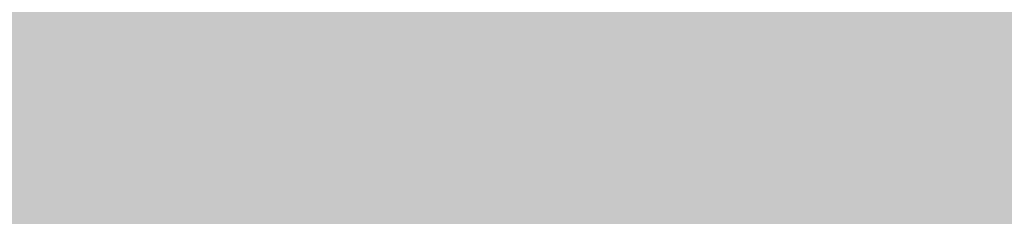
# Model space of a CAD drawing. Units: millimetres. Extents: x -22994 to 29398, y -19990 to 20176.
# Tile 94 of 135: x 229.428 to 230.597, y 84.264 to 84.498. Entities that reach past the tile are written whole.
import ezdxf
from ezdxf import colors
from ezdxf.entities.mleader import LeaderData, LeaderLine
from ezdxf.math import Vec2, Vec3

# ---------------------------------------------------------------- set-up
doc = ezdxf.new("R2010")
doc.units = ezdxf.units.MM
doc.header["$MEASUREMENT"] = 0
for name, color, linetype, lineweight in [('M-ANNO-TEXT', 7, 'Continuous', 25), ('M-DIMS', 2, 'Continuous', 18), ('M-EQPM-PATT', 7, 'Continuous', 18)]:
    doc.layers.add(name, color=color, linetype=linetype, lineweight=lineweight)
doc.styles.get("Standard").update_dxf_attribs({"font": 'arial.ttf'})
doc.dimstyles.get("Standard").update_dxf_attribs({"dimtxt": 0.18, "dimasz": 10000, "dimexe": 0.18, "dimexo": 0.0625, "dimgap": 0.09, "dimtad": 0, "dimtih": 1, "dimtoh": 1, "dimdec": 0, "dimzin": 0, "dimdsep": 46, "dimtxsty": 'Standard', "dimcen": 0.09, "dimadec": 0, "dimazin": 0, "dimtfac": 1, "dimtdec": 0, "dimtofl": 0, "dimtmove": 0, "dimatfit": 3, "dimfxl": 1, "dimtolj": 1, "dimtzin": 0, "dimlwd": 30, "dimarcsym": 0})

# ---------------------------------------------------------------- blocks, each defined once
blk = doc.blocks.new('*D2')
at = {"layer": 'Defpoints', "color": 0, "transparency": 16777216}
for p in [(6.6773, 10.2713), (290.852, 10.2713), (290.852, -5.0787)]:
    blk.add_point(p, dxfattribs=at)
at = {"layer": 'M-DIMS', "color": 0, "lineweight": -2, "transparency": 16777216}
for p, q in [((6.6773, 10.2088), (6.6773, -5.2587)), ((290.852, 10.2088), (290.852, -5.2587))]:
    blk.add_line(p, q, dxfattribs=at)
at = {"layer": 'M-DIMS', "color": 0, "lineweight": 30, "transparency": 16777216}
for p, q in [((-9993.3227, -5.0787), (-19993.3227, -5.0787)), ((10290.852, -5.0787), (20290.852, -5.0787))]:
    blk.add_line(p, q, dxfattribs=at)
at = {"layer": 'M-DIMS', "color": 0, "transparency": 16777216}
for points in [[(-9993.3227, 1661.5879), (-9993.3227, -1671.7454), (6.6773, -5.0787)], [(10290.852, 1661.5879), (10290.852, -1671.7454), (290.852, -5.0787)]]:
    blk.add_solid(points, dxfattribs=at)
at = {"layer": 'M-DIMS', "color": 0, "transparency": 16777216, "insert": (148.7647, -5.0787), "char_height": 0.18, "attachment_point": 5}
blk.add_mtext('\\A1;284.2', dxfattribs=at)
blk = doc.blocks.new('*D3')
at = {"layer": 'Defpoints', "color": 0, "transparency": 16777216}
for p in [(110.2647, 204.1654), (110.2647, 176.3662), (95.8327, 127.967)]:
    blk.add_point(p, dxfattribs=at)
at = {"layer": 'M-DIMS', "color": 0, "lineweight": -2, "transparency": 16777216}
for p, q in [((95.8327, 128.0295), (95.8327, 204.3454)), ((110.2647, 176.4287), (110.2647, 204.3454))]:
    blk.add_line(p, q, dxfattribs=at)
at = {"layer": 'M-DIMS', "color": 0, "lineweight": 30, "transparency": 16777216}
for p, q in [((-9904.1673, 204.1654), (-19904.1673, 204.1654)), ((10110.2647, 204.1654), (20110.2647, 204.1654))]:
    blk.add_line(p, q, dxfattribs=at)
at = {"layer": 'M-DIMS', "color": 0, "transparency": 16777216}
for points in [[(-9904.1673, 1870.8321), (-9904.1673, -1462.5013), (95.8327, 204.1654)], [(10110.2647, 1870.8321), (10110.2647, -1462.5013), (110.2647, 204.1654)]]:
    blk.add_solid(points, dxfattribs=at)
at = {"layer": 'M-DIMS', "color": 0, "transparency": 16777216, "insert": (103.0487, 204.1654), "char_height": 0.18, "attachment_point": 5}
blk.add_mtext('\\A1;14.432', dxfattribs=at)
blk = doc.blocks.new('*D4')
at = {"layer": 'Defpoints', "color": 0, "transparency": 16777216}
for p in [(116.2647, 204.1654), (110.2647, 176.3662), (116.2647, 176.3662)]:
    blk.add_point(p, dxfattribs=at)
at = {"layer": 'M-DIMS', "color": 0, "lineweight": -2, "transparency": 16777216}
for p, q in [((110.2647, 176.4287), (110.2647, 204.3454)), ((116.2647, 176.4287), (116.2647, 204.3454))]:
    blk.add_line(p, q, dxfattribs=at)
at = {"layer": 'M-DIMS', "color": 0, "lineweight": 30, "transparency": 16777216}
for p, q in [((-9889.7353, 204.1654), (-19889.7353, 204.1654)), ((10116.2647, 204.1654), (20116.2647, 204.1654))]:
    blk.add_line(p, q, dxfattribs=at)
at = {"layer": 'M-DIMS', "color": 0, "transparency": 16777216}
for points in [[(-9889.7353, 1870.8321), (-9889.7353, -1462.5013), (110.2647, 204.1654)], [(10116.2647, 1870.8321), (10116.2647, -1462.5013), (116.2647, 204.1654)]]:
    blk.add_solid(points, dxfattribs=at)
at = {"layer": 'M-DIMS', "color": 0, "transparency": 16777216, "insert": (113.2647, 204.1654), "char_height": 0.18, "attachment_point": 5}
blk.add_mtext('\\A1;6', dxfattribs=at)
blk = doc.blocks.new('*D5')
at = {"layer": 'Defpoints', "color": 0, "transparency": 16777216}
for p in [(181.2647, 204.1654), (116.2647, 176.3662), (181.2647, 176.3662)]:
    blk.add_point(p, dxfattribs=at)
at = {"layer": 'M-DIMS', "color": 0, "lineweight": -2, "transparency": 16777216}
for p, q in [((116.2647, 176.4287), (116.2647, 204.3454)), ((181.2647, 176.4287), (181.2647, 204.3454))]:
    blk.add_line(p, q, dxfattribs=at)
at = {"layer": 'M-DIMS', "color": 0, "lineweight": 30, "transparency": 16777216}
for p, q in [((-9883.7353, 204.1654), (-19883.7353, 204.1654)), ((10181.2647, 204.1654), (20181.2647, 204.1654))]:
    blk.add_line(p, q, dxfattribs=at)
at = {"layer": 'M-DIMS', "color": 0, "transparency": 16777216}
for points in [[(-9883.7353, 1870.8321), (-9883.7353, -1462.5013), (116.2647, 204.1654)], [(10181.2647, 1870.8321), (10181.2647, -1462.5013), (181.2647, 204.1654)]]:
    blk.add_solid(points, dxfattribs=at)
at = {"layer": 'M-DIMS', "color": 0, "transparency": 16777216, "insert": (148.7647, 204.1654), "char_height": 0.18, "attachment_point": 5}
blk.add_mtext('\\A1;65', dxfattribs=at)
blk = doc.blocks.new('*D6')
at = {"layer": 'Defpoints', "color": 0, "transparency": 16777216}
for p in [(187.2647, 204.1654), (181.2647, 176.3662), (187.2647, 176.3662)]:
    blk.add_point(p, dxfattribs=at)
at = {"layer": 'M-DIMS', "color": 0, "lineweight": -2, "transparency": 16777216}
for p, q in [((181.2647, 176.4287), (181.2647, 204.3454)), ((187.2647, 176.4287), (187.2647, 204.3454))]:
    blk.add_line(p, q, dxfattribs=at)
at = {"layer": 'M-DIMS', "color": 0, "lineweight": 30, "transparency": 16777216}
for p, q in [((-9818.7353, 204.1654), (-19818.7353, 204.1654)), ((10187.2647, 204.1654), (20187.2647, 204.1654))]:
    blk.add_line(p, q, dxfattribs=at)
at = {"layer": 'M-DIMS', "color": 0, "transparency": 16777216}
for points in [[(-9818.7353, 1870.8321), (-9818.7353, -1462.5013), (181.2647, 204.1654)], [(10187.2647, 1870.8321), (10187.2647, -1462.5013), (187.2647, 204.1654)]]:
    blk.add_solid(points, dxfattribs=at)
at = {"layer": 'M-DIMS', "color": 0, "transparency": 16777216, "insert": (184.2647, 204.1654), "char_height": 0.18, "attachment_point": 5}
blk.add_mtext('\\A1;6', dxfattribs=at)
blk = doc.blocks.new('*D7')
at = {"layer": 'Defpoints', "color": 0, "transparency": 16777216}
for p in [(201.6967, 204.1654), (187.2647, 176.3662), (201.6967, 127.967)]:
    blk.add_point(p, dxfattribs=at)
at = {"layer": 'M-DIMS', "color": 0, "lineweight": -2, "transparency": 16777216}
for p, q in [((187.2647, 176.4287), (187.2647, 204.3454)), ((201.6967, 128.0295), (201.6967, 204.3454))]:
    blk.add_line(p, q, dxfattribs=at)
at = {"layer": 'M-DIMS', "color": 0, "lineweight": 30, "transparency": 16777216}
for p, q in [((-9812.7353, 204.1654), (-19812.7353, 204.1654)), ((10201.6967, 204.1654), (20201.6967, 204.1654))]:
    blk.add_line(p, q, dxfattribs=at)
at = {"layer": 'M-DIMS', "color": 0, "transparency": 16777216}
for points in [[(-9812.7353, 1870.8321), (-9812.7353, -1462.5013), (187.2647, 204.1654)], [(10201.6967, 1870.8321), (10201.6967, -1462.5013), (201.6967, 204.1654)]]:
    blk.add_solid(points, dxfattribs=at)
at = {"layer": 'M-DIMS', "color": 0, "transparency": 16777216, "insert": (194.4807, 204.1654), "char_height": 0.18, "attachment_point": 5}
blk.add_mtext('\\A1;14.432', dxfattribs=at)
blk = doc.blocks.new('*D8')
at = {"layer": 'Defpoints', "color": 0, "transparency": 16777216}
for p in [(227.6485, 204.1654), (227.6485, 146.7296), (201.6967, 127.967)]:
    blk.add_point(p, dxfattribs=at)
at = {"layer": 'M-DIMS', "color": 0, "lineweight": -2, "transparency": 16777216}
for p, q in [((201.6967, 128.0295), (201.6967, 204.3454)), ((227.6485, 146.7921), (227.6485, 204.3454))]:
    blk.add_line(p, q, dxfattribs=at)
at = {"layer": 'M-DIMS', "color": 0, "lineweight": 30, "transparency": 16777216}
for p, q in [((-9798.3033, 204.1654), (-19798.3033, 204.1654)), ((10227.6485, 204.1654), (20227.6485, 204.1654))]:
    blk.add_line(p, q, dxfattribs=at)
at = {"layer": 'M-DIMS', "color": 0, "transparency": 16777216}
for points in [[(-9798.3033, 1870.8321), (-9798.3033, -1462.5013), (201.6967, 204.1654)], [(10227.6485, 1870.8321), (10227.6485, -1462.5013), (227.6485, 204.1654)]]:
    blk.add_solid(points, dxfattribs=at)
at = {"layer": 'M-DIMS', "color": 0, "transparency": 16777216, "insert": (214.6726, 204.1654), "char_height": 0.18, "attachment_point": 5}
blk.add_mtext('\\A1;25.95', dxfattribs=at)
blk = doc.blocks.new('*D9')
at = {"layer": 'Defpoints', "color": 0, "transparency": 16777216}
for p in [(187.2647, 176.3662), (306.202, 176.3662), (290.852, 10.2713)]:
    blk.add_point(p, dxfattribs=at)
at = {"layer": 'M-DIMS', "color": 0, "lineweight": 30, "transparency": 16777216}
for p, q in [((306.202, 10176.3662), (306.202, 20176.3662)), ((306.202, -9989.7287), (306.202, -19989.7287))]:
    blk.add_line(p, q, dxfattribs=at)
at = {"layer": 'M-DIMS', "color": 0, "lineweight": -2, "transparency": 16777216}
for p, q in [((187.3272, 176.3662), (306.382, 176.3662)), ((290.9145, 10.2713), (306.382, 10.2713))]:
    blk.add_line(p, q, dxfattribs=at)
at = {"layer": 'M-DIMS', "color": 0, "transparency": 16777216}
for points in [[(-1360.4646, 10176.3662), (1972.8687, 10176.3662), (306.202, 176.3662)], [(-1360.4646, -9989.7287), (1972.8687, -9989.7287), (306.202, 10.2713)]]:
    blk.add_solid(points, dxfattribs=at)
at = {"layer": 'M-DIMS', "color": 0, "transparency": 16777216, "insert": (306.202, 93.3187), "char_height": 0.18, "attachment_point": 5}
blk.add_mtext('\\A1;166.1', dxfattribs=at)
blk = doc.blocks.new('*D10')
at = {"layer": 'Defpoints', "color": 0, "transparency": 16777216}
for p in [(125.6498, 136.0713), (133.3459, 136.0713), (133.3459, -5.0787)]:
    blk.add_point(p, dxfattribs=at)
at = {"layer": 'M-DIMS', "color": 0, "lineweight": -2, "transparency": 16777216}
for p, q in [((125.6498, 136.0088), (125.6498, -5.2587)), ((133.3459, 136.0088), (133.3459, -5.2587))]:
    blk.add_line(p, q, dxfattribs=at)
at = {"layer": 'M-DIMS', "color": 0, "lineweight": 30, "transparency": 16777216}
for p, q in [((-9874.3502, -5.0787), (-19874.3502, -5.0787)), ((10133.3459, -5.0787), (20133.3459, -5.0787))]:
    blk.add_line(p, q, dxfattribs=at)
at = {"layer": 'M-DIMS', "color": 0, "transparency": 16777216}
for points in [[(-9874.3502, 1661.5879), (-9874.3502, -1671.7454), (125.6498, -5.0787)], [(10133.3459, 1661.5879), (10133.3459, -1671.7454), (133.3459, -5.0787)]]:
    blk.add_solid(points, dxfattribs=at)
at = {"layer": 'M-DIMS', "color": 0, "transparency": 16777216, "insert": (129.4978, -5.0787), "char_height": 0.18, "attachment_point": 5}
blk.add_mtext('\\A1;7.696', dxfattribs=at)
blk = doc.blocks.new('*D11')
at = {"layer": 'Defpoints', "color": 0, "transparency": 16777216}
for p in [(133.3459, 136.0713), (135.6498, 136.0713), (135.6498, -5.0787)]:
    blk.add_point(p, dxfattribs=at)
at = {"layer": 'M-DIMS', "color": 0, "lineweight": -2, "transparency": 16777216}
for p, q in [((133.3459, 136.0088), (133.3459, -5.2587)), ((135.6498, 136.0088), (135.6498, -5.2587))]:
    blk.add_line(p, q, dxfattribs=at)
at = {"layer": 'M-DIMS', "color": 0, "lineweight": 30, "transparency": 16777216}
for p, q in [((-9866.6541, -5.0787), (-19866.6541, -5.0787)), ((10135.6498, -5.0787), (20135.6498, -5.0787))]:
    blk.add_line(p, q, dxfattribs=at)
at = {"layer": 'M-DIMS', "color": 0, "transparency": 16777216}
for points in [[(-9866.6541, 1661.5879), (-9866.6541, -1671.7454), (133.3459, -5.0787)], [(10135.6498, 1661.5879), (10135.6498, -1671.7454), (135.6498, -5.0787)]]:
    blk.add_solid(points, dxfattribs=at)
at = {"layer": 'M-DIMS', "color": 0, "transparency": 16777216, "insert": (134.4978, -5.0787), "char_height": 0.18, "attachment_point": 5}
blk.add_mtext('\\A1;2.304', dxfattribs=at)
blk = doc.blocks.new('*D12')
at = {"layer": 'Defpoints', "color": 0, "transparency": 16777216}
for p in [(135.6498, 136.0713), (145.6498, 136.0713), (145.6498, -5.0787)]:
    blk.add_point(p, dxfattribs=at)
at = {"layer": 'M-DIMS', "color": 0, "lineweight": -2, "transparency": 16777216}
for p, q in [((135.6498, 136.0088), (135.6498, -5.2587)), ((145.6498, 136.0088), (145.6498, -5.2587))]:
    blk.add_line(p, q, dxfattribs=at)
at = {"layer": 'M-DIMS', "color": 0, "lineweight": 30, "transparency": 16777216}
for p, q in [((-9864.3502, -5.0787), (-19864.3502, -5.0787)), ((10145.6498, -5.0787), (20145.6498, -5.0787))]:
    blk.add_line(p, q, dxfattribs=at)
at = {"layer": 'M-DIMS', "color": 0, "transparency": 16777216}
for points in [[(-9864.3502, 1661.5879), (-9864.3502, -1671.7454), (135.6498, -5.0787)], [(10145.6498, 1661.5879), (10145.6498, -1671.7454), (145.6498, -5.0787)]]:
    blk.add_solid(points, dxfattribs=at)
at = {"layer": 'M-DIMS', "color": 0, "transparency": 16777216, "insert": (140.6498, -5.0787), "char_height": 0.18, "attachment_point": 5}
blk.add_mtext('\\A1;10', dxfattribs=at)
blk = doc.blocks.new('*D13')
at = {"layer": 'Defpoints', "color": 0, "transparency": 16777216}
for p in [(145.6498, 136.0713), (155.6498, 136.0713), (155.6498, -5.0787)]:
    blk.add_point(p, dxfattribs=at)
at = {"layer": 'M-DIMS', "color": 0, "lineweight": -2, "transparency": 16777216}
for p, q in [((145.6498, 136.0088), (145.6498, -5.2587)), ((155.6498, 136.0088), (155.6498, -5.2587))]:
    blk.add_line(p, q, dxfattribs=at)
at = {"layer": 'M-DIMS', "color": 0, "lineweight": 30, "transparency": 16777216}
for p, q in [((-9854.3502, -5.0787), (-19854.3502, -5.0787)), ((10155.6498, -5.0787), (20155.6498, -5.0787))]:
    blk.add_line(p, q, dxfattribs=at)
at = {"layer": 'M-DIMS', "color": 0, "transparency": 16777216}
for points in [[(-9854.3502, 1661.5879), (-9854.3502, -1671.7454), (145.6498, -5.0787)], [(10155.6498, 1661.5879), (10155.6498, -1671.7454), (155.6498, -5.0787)]]:
    blk.add_solid(points, dxfattribs=at)
at = {"layer": 'M-DIMS', "color": 0, "transparency": 16777216, "insert": (150.6498, -5.0787), "char_height": 0.18, "attachment_point": 5}
blk.add_mtext('\\A1;10', dxfattribs=at)
blk = doc.blocks.new('*D14')
at = {"layer": 'Defpoints', "color": 0, "transparency": 16777216}
for p in [(155.6498, 136.0713), (165.6498, 136.0713), (165.6498, -5.0787)]:
    blk.add_point(p, dxfattribs=at)
at = {"layer": 'M-DIMS', "color": 0, "lineweight": -2, "transparency": 16777216}
for p, q in [((155.6498, 136.0088), (155.6498, -5.2587)), ((165.6498, 136.0088), (165.6498, -5.2587))]:
    blk.add_line(p, q, dxfattribs=at)
at = {"layer": 'M-DIMS', "color": 0, "lineweight": 30, "transparency": 16777216}
for p, q in [((-9844.3502, -5.0787), (-19844.3502, -5.0787)), ((10165.6498, -5.0787), (20165.6498, -5.0787))]:
    blk.add_line(p, q, dxfattribs=at)
at = {"layer": 'M-DIMS', "color": 0, "transparency": 16777216}
for points in [[(-9844.3502, 1661.5879), (-9844.3502, -1671.7454), (155.6498, -5.0787)], [(10165.6498, 1661.5879), (10165.6498, -1671.7454), (165.6498, -5.0787)]]:
    blk.add_solid(points, dxfattribs=at)
at = {"layer": 'M-DIMS', "color": 0, "transparency": 16777216, "insert": (160.6498, -5.0787), "char_height": 0.18, "attachment_point": 5}
blk.add_mtext('\\A1;10', dxfattribs=at)
blk = doc.blocks.new('*D15')
at = {"layer": 'Defpoints', "color": 0, "transparency": 16777216}
for p in [(173.3459, 154.788), (173.3459, 136.0713), (306.202, 136.0713)]:
    blk.add_point(p, dxfattribs=at)
at = {"layer": 'M-DIMS', "color": 0, "lineweight": 30, "transparency": 16777216}
for p, q in [((306.202, 10154.788), (306.202, 20154.788)), ((306.202, -9863.9287), (306.202, -19863.9287))]:
    blk.add_line(p, q, dxfattribs=at)
at = {"layer": 'M-DIMS', "color": 0, "lineweight": -2, "transparency": 16777216}
for p, q in [((173.4084, 154.788), (306.382, 154.788)), ((173.4084, 136.0713), (306.382, 136.0713))]:
    blk.add_line(p, q, dxfattribs=at)
at = {"layer": 'M-DIMS', "color": 0, "transparency": 16777216}
for points in [[(-1360.4646, 10154.788), (1972.8687, 10154.788), (306.202, 154.788)], [(-1360.4646, -9863.9287), (1972.8687, -9863.9287), (306.202, 136.0713)]]:
    blk.add_solid(points, dxfattribs=at)
at = {"layer": 'M-DIMS', "color": 0, "transparency": 16777216, "insert": (306.202, 145.4297), "char_height": 0.18, "attachment_point": 5}
blk.add_mtext('\\A1;18.717', dxfattribs=at)
blk = doc.blocks.new('*D16')
at = {"layer": 'Defpoints', "color": 0, "transparency": 16777216}
for p in [(120.1702, 204.1654), (110.4658, 48.0349), (120.1702, 48.0349)]:
    blk.add_point(p, dxfattribs=at)
at = {"layer": 'M-DIMS', "color": 0, "lineweight": -2, "transparency": 16777216}
for p, q in [((110.4658, 48.0974), (110.4658, 204.3454)), ((120.1702, 48.0974), (120.1702, 204.3454))]:
    blk.add_line(p, q, dxfattribs=at)
at = {"layer": 'M-DIMS', "color": 0, "lineweight": 30, "transparency": 16777216}
for p, q in [((-9889.5342, 204.1654), (-19889.5342, 204.1654)), ((10120.1702, 204.1654), (20120.1702, 204.1654))]:
    blk.add_line(p, q, dxfattribs=at)
at = {"layer": 'M-DIMS', "color": 0, "transparency": 16777216}
for points in [[(-9889.5342, 1870.8321), (-9889.5342, -1462.5013), (110.4658, 204.1654)], [(10120.1702, 1870.8321), (10120.1702, -1462.5013), (120.1702, 204.1654)]]:
    blk.add_solid(points, dxfattribs=at)
at = {"layer": 'M-DIMS', "color": 0, "transparency": 16777216, "insert": (115.318, 204.1654), "char_height": 0.18, "attachment_point": 5}
blk.add_mtext('\\A1;9.704', dxfattribs=at)
blk = doc.blocks.new('*D17')
at = {"layer": 'Defpoints', "color": 0, "transparency": 16777216}
for p in [(126.1702, 204.1654), (120.1702, 48.0349), (126.1702, 48.0349)]:
    blk.add_point(p, dxfattribs=at)
at = {"layer": 'M-DIMS', "color": 0, "lineweight": -2, "transparency": 16777216}
for p, q in [((120.1702, 48.0974), (120.1702, 204.3454)), ((126.1702, 48.0974), (126.1702, 204.3454))]:
    blk.add_line(p, q, dxfattribs=at)
at = {"layer": 'M-DIMS', "color": 0, "lineweight": 30, "transparency": 16777216}
for p, q in [((-9879.8298, 204.1654), (-19879.8298, 204.1654)), ((10126.1702, 204.1654), (20126.1702, 204.1654))]:
    blk.add_line(p, q, dxfattribs=at)
at = {"layer": 'M-DIMS', "color": 0, "transparency": 16777216}
for points in [[(-9879.8298, 1870.8321), (-9879.8298, -1462.5013), (120.1702, 204.1654)], [(10126.1702, 1870.8321), (10126.1702, -1462.5013), (126.1702, 204.1654)]]:
    blk.add_solid(points, dxfattribs=at)
at = {"layer": 'M-DIMS', "color": 0, "transparency": 16777216, "insert": (123.1702, 204.1654), "char_height": 0.18, "attachment_point": 5}
blk.add_mtext('\\A1;6', dxfattribs=at)
blk = doc.blocks.new('*D18')
at = {"layer": 'Defpoints', "color": 0, "transparency": 16777216}
for p in [(132.1702, 204.1654), (126.1702, 48.0349), (132.1702, 48.0349)]:
    blk.add_point(p, dxfattribs=at)
at = {"layer": 'M-DIMS', "color": 0, "lineweight": -2, "transparency": 16777216}
for p, q in [((126.1702, 48.0974), (126.1702, 204.3454)), ((132.1702, 48.0974), (132.1702, 204.3454))]:
    blk.add_line(p, q, dxfattribs=at)
at = {"layer": 'M-DIMS', "color": 0, "lineweight": 30, "transparency": 16777216}
for p, q in [((-9873.8298, 204.1654), (-19873.8298, 204.1654)), ((10132.1702, 204.1654), (20132.1702, 204.1654))]:
    blk.add_line(p, q, dxfattribs=at)
at = {"layer": 'M-DIMS', "color": 0, "transparency": 16777216}
for points in [[(-9873.8298, 1870.8321), (-9873.8298, -1462.5013), (126.1702, 204.1654)], [(10132.1702, 1870.8321), (10132.1702, -1462.5013), (132.1702, 204.1654)]]:
    blk.add_solid(points, dxfattribs=at)
at = {"layer": 'M-DIMS', "color": 0, "transparency": 16777216, "insert": (129.1702, 204.1654), "char_height": 0.18, "attachment_point": 5}
blk.add_mtext('\\A1;6', dxfattribs=at)
blk = doc.blocks.new('*D19')
at = {"layer": 'Defpoints', "color": 0, "transparency": 16777216}
for p in [(138.1702, 204.1654), (132.1702, 48.0349), (138.1702, 48.0349)]:
    blk.add_point(p, dxfattribs=at)
at = {"layer": 'M-DIMS', "color": 0, "lineweight": -2, "transparency": 16777216}
for p, q in [((132.1702, 48.0974), (132.1702, 204.3454)), ((138.1702, 48.0974), (138.1702, 204.3454))]:
    blk.add_line(p, q, dxfattribs=at)
at = {"layer": 'M-DIMS', "color": 0, "lineweight": 30, "transparency": 16777216}
for p, q in [((-9867.8298, 204.1654), (-19867.8298, 204.1654)), ((10138.1702, 204.1654), (20138.1702, 204.1654))]:
    blk.add_line(p, q, dxfattribs=at)
at = {"layer": 'M-DIMS', "color": 0, "transparency": 16777216}
for points in [[(-9867.8298, 1870.8321), (-9867.8298, -1462.5013), (132.1702, 204.1654)], [(10138.1702, 1870.8321), (10138.1702, -1462.5013), (138.1702, 204.1654)]]:
    blk.add_solid(points, dxfattribs=at)
at = {"layer": 'M-DIMS', "color": 0, "transparency": 16777216, "insert": (135.1702, 204.1654), "char_height": 0.18, "attachment_point": 5}
blk.add_mtext('\\A1;6', dxfattribs=at)
blk = doc.blocks.new('*D20')
at = {"layer": 'Defpoints', "color": 0, "transparency": 16777216}
for p in [(144.1702, 204.1654), (138.1702, 48.0349), (144.1702, 48.0349)]:
    blk.add_point(p, dxfattribs=at)
at = {"layer": 'M-DIMS', "color": 0, "lineweight": -2, "transparency": 16777216}
for p, q in [((138.1702, 48.0974), (138.1702, 204.3454)), ((144.1702, 48.0974), (144.1702, 204.3454))]:
    blk.add_line(p, q, dxfattribs=at)
at = {"layer": 'M-DIMS', "color": 0, "lineweight": 30, "transparency": 16777216}
for p, q in [((-9861.8298, 204.1654), (-19861.8298, 204.1654)), ((10144.1702, 204.1654), (20144.1702, 204.1654))]:
    blk.add_line(p, q, dxfattribs=at)
at = {"layer": 'M-DIMS', "color": 0, "transparency": 16777216}
for points in [[(-9861.8298, 1870.8321), (-9861.8298, -1462.5013), (138.1702, 204.1654)], [(10144.1702, 1870.8321), (10144.1702, -1462.5013), (144.1702, 204.1654)]]:
    blk.add_solid(points, dxfattribs=at)
at = {"layer": 'M-DIMS', "color": 0, "transparency": 16777216, "insert": (141.1702, 204.1654), "char_height": 0.18, "attachment_point": 5}
blk.add_mtext('\\A1;6', dxfattribs=at)
blk = doc.blocks.new('*D21')
at = {"layer": 'Defpoints', "color": 0, "transparency": 16777216}
for p in [(149.1157, 204.1654), (144.1702, 48.0349), (149.1157, 48.0349)]:
    blk.add_point(p, dxfattribs=at)
at = {"layer": 'M-DIMS', "color": 0, "lineweight": -2, "transparency": 16777216}
for p, q in [((144.1702, 48.0974), (144.1702, 204.3454)), ((149.1157, 48.0974), (149.1157, 204.3454))]:
    blk.add_line(p, q, dxfattribs=at)
at = {"layer": 'M-DIMS', "color": 0, "lineweight": 30, "transparency": 16777216}
for p, q in [((-9855.8298, 204.1654), (-19855.8298, 204.1654)), ((10149.1157, 204.1654), (20149.1157, 204.1654))]:
    blk.add_line(p, q, dxfattribs=at)
at = {"layer": 'M-DIMS', "color": 0, "transparency": 16777216}
for points in [[(-9855.8298, 1870.8321), (-9855.8298, -1462.5013), (144.1702, 204.1654)], [(10149.1157, 1870.8321), (10149.1157, -1462.5013), (149.1157, 204.1654)]]:
    blk.add_solid(points, dxfattribs=at)
at = {"layer": 'M-DIMS', "color": 0, "transparency": 16777216, "insert": (146.6429, 204.1654), "char_height": 0.18, "attachment_point": 5}
blk.add_mtext('\\A1;4.945', dxfattribs=at)
blk = doc.blocks.new('*D22')
at = {"layer": 'Defpoints', "color": 0, "transparency": 16777216}
for p in [(149.1157, 30.9895), (155.1157, 30.9895), (155.1157, -5.0787)]:
    blk.add_point(p, dxfattribs=at)
at = {"layer": 'M-DIMS', "color": 0, "lineweight": -2, "transparency": 16777216}
for p, q in [((149.1157, 30.927), (149.1157, -5.2587)), ((155.1157, 30.927), (155.1157, -5.2587))]:
    blk.add_line(p, q, dxfattribs=at)
at = {"layer": 'M-DIMS', "color": 0, "lineweight": 30, "transparency": 16777216}
for p, q in [((-9850.8843, -5.0787), (-19850.8843, -5.0787)), ((10155.1157, -5.0787), (20155.1157, -5.0787))]:
    blk.add_line(p, q, dxfattribs=at)
at = {"layer": 'M-DIMS', "color": 0, "transparency": 16777216}
for points in [[(-9850.8843, 1661.5879), (-9850.8843, -1671.7454), (149.1157, -5.0787)], [(10155.1157, 1661.5879), (10155.1157, -1671.7454), (155.1157, -5.0787)]]:
    blk.add_solid(points, dxfattribs=at)
at = {"layer": 'M-DIMS', "color": 0, "transparency": 16777216, "insert": (152.1157, -5.0787), "char_height": 0.18, "attachment_point": 5}
blk.add_mtext('\\A1;6', dxfattribs=at)
blk = doc.blocks.new('*D23')
at = {"layer": 'Defpoints', "color": 0, "transparency": 16777216}
for p in [(155.1157, 30.9895), (161.1157, 30.9895), (161.1157, -5.0787)]:
    blk.add_point(p, dxfattribs=at)
at = {"layer": 'M-DIMS', "color": 0, "lineweight": -2, "transparency": 16777216}
for p, q in [((155.1157, 30.927), (155.1157, -5.2587)), ((161.1157, 30.927), (161.1157, -5.2587))]:
    blk.add_line(p, q, dxfattribs=at)
at = {"layer": 'M-DIMS', "color": 0, "lineweight": 30, "transparency": 16777216}
for p, q in [((-9844.8843, -5.0787), (-19844.8843, -5.0787)), ((10161.1157, -5.0787), (20161.1157, -5.0787))]:
    blk.add_line(p, q, dxfattribs=at)
at = {"layer": 'M-DIMS', "color": 0, "transparency": 16777216}
for points in [[(-9844.8843, 1661.5879), (-9844.8843, -1671.7454), (155.1157, -5.0787)], [(10161.1157, 1661.5879), (10161.1157, -1671.7454), (161.1157, -5.0787)]]:
    blk.add_solid(points, dxfattribs=at)
at = {"layer": 'M-DIMS', "color": 0, "transparency": 16777216, "insert": (158.1157, -5.0787), "char_height": 0.18, "attachment_point": 5}
blk.add_mtext('\\A1;6', dxfattribs=at)
blk = doc.blocks.new('*D24')
at = {"layer": 'Defpoints', "color": 0, "transparency": 16777216}
for p in [(161.1157, 30.9895), (166.4387, 30.9895), (166.4387, -5.0787)]:
    blk.add_point(p, dxfattribs=at)
at = {"layer": 'M-DIMS', "color": 0, "lineweight": -2, "transparency": 16777216}
for p, q in [((161.1157, 30.927), (161.1157, -5.2587)), ((166.4387, 30.927), (166.4387, -5.2587))]:
    blk.add_line(p, q, dxfattribs=at)
at = {"layer": 'M-DIMS', "color": 0, "lineweight": 30, "transparency": 16777216}
for p, q in [((-9838.8843, -5.0787), (-19838.8843, -5.0787)), ((10166.4387, -5.0787), (20166.4387, -5.0787))]:
    blk.add_line(p, q, dxfattribs=at)
at = {"layer": 'M-DIMS', "color": 0, "transparency": 16777216}
for points in [[(-9838.8843, 1661.5879), (-9838.8843, -1671.7454), (161.1157, -5.0787)], [(10166.4387, 1661.5879), (10166.4387, -1671.7454), (166.4387, -5.0787)]]:
    blk.add_solid(points, dxfattribs=at)
at = {"layer": 'M-DIMS', "color": 0, "transparency": 16777216, "insert": (163.7772, -5.0787), "char_height": 0.18, "attachment_point": 5}
blk.add_mtext('\\A1;5.323', dxfattribs=at)
blk = doc.blocks.new('*D25')
at = {"layer": 'Defpoints', "color": 0, "transparency": 16777216}
for p in [(166.4387, 30.9895), (172.4387, 30.9895), (172.4387, -5.0787)]:
    blk.add_point(p, dxfattribs=at)
at = {"layer": 'M-DIMS', "color": 0, "lineweight": -2, "transparency": 16777216}
for p, q in [((166.4387, 30.927), (166.4387, -5.2587)), ((172.4387, 30.927), (172.4387, -5.2587))]:
    blk.add_line(p, q, dxfattribs=at)
at = {"layer": 'M-DIMS', "color": 0, "lineweight": 30, "transparency": 16777216}
for p, q in [((-9833.5613, -5.0787), (-19833.5613, -5.0787)), ((10172.4387, -5.0787), (20172.4387, -5.0787))]:
    blk.add_line(p, q, dxfattribs=at)
at = {"layer": 'M-DIMS', "color": 0, "transparency": 16777216}
for points in [[(-9833.5613, 1661.5879), (-9833.5613, -1671.7454), (166.4387, -5.0787)], [(10172.4387, 1661.5879), (10172.4387, -1671.7454), (172.4387, -5.0787)]]:
    blk.add_solid(points, dxfattribs=at)
at = {"layer": 'M-DIMS', "color": 0, "transparency": 16777216, "insert": (169.4387, -5.0787), "char_height": 0.18, "attachment_point": 5}
blk.add_mtext('\\A1;6', dxfattribs=at)
blk = doc.blocks.new('*D26')
at = {"layer": 'Defpoints', "color": 0, "transparency": 16777216}
for p in [(172.4387, 30.9895), (178.4387, 30.9895), (178.4387, -5.0787)]:
    blk.add_point(p, dxfattribs=at)
at = {"layer": 'M-DIMS', "color": 0, "lineweight": -2, "transparency": 16777216}
for p, q in [((172.4387, 30.927), (172.4387, -5.2587)), ((178.4387, 30.927), (178.4387, -5.2587))]:
    blk.add_line(p, q, dxfattribs=at)
at = {"layer": 'M-DIMS', "color": 0, "lineweight": 30, "transparency": 16777216}
for p, q in [((-9827.5613, -5.0787), (-19827.5613, -5.0787)), ((10178.4387, -5.0787), (20178.4387, -5.0787))]:
    blk.add_line(p, q, dxfattribs=at)
at = {"layer": 'M-DIMS', "color": 0, "transparency": 16777216}
for points in [[(-9827.5613, 1661.5879), (-9827.5613, -1671.7454), (172.4387, -5.0787)], [(10178.4387, 1661.5879), (10178.4387, -1671.7454), (178.4387, -5.0787)]]:
    blk.add_solid(points, dxfattribs=at)
at = {"layer": 'M-DIMS', "color": 0, "transparency": 16777216, "insert": (175.4387, -5.0787), "char_height": 0.18, "attachment_point": 5}
blk.add_mtext('\\A1;6', dxfattribs=at)
blk = doc.blocks.new('*D27')
at = {"layer": 'Defpoints', "color": 0, "transparency": 16777216}
for p in [(178.4387, 30.9895), (188.1175, 30.9895), (188.1175, -5.0787)]:
    blk.add_point(p, dxfattribs=at)
at = {"layer": 'M-DIMS', "color": 0, "lineweight": -2, "transparency": 16777216}
for p, q in [((178.4387, 30.927), (178.4387, -5.2587)), ((188.1175, 30.927), (188.1175, -5.2587))]:
    blk.add_line(p, q, dxfattribs=at)
at = {"layer": 'M-DIMS', "color": 0, "lineweight": 30, "transparency": 16777216}
for p, q in [((-9821.5613, -5.0787), (-19821.5613, -5.0787)), ((10188.1175, -5.0787), (20188.1175, -5.0787))]:
    blk.add_line(p, q, dxfattribs=at)
at = {"layer": 'M-DIMS', "color": 0, "transparency": 16777216}
for points in [[(-9821.5613, 1661.5879), (-9821.5613, -1671.7454), (178.4387, -5.0787)], [(10188.1175, 1661.5879), (10188.1175, -1671.7454), (188.1175, -5.0787)]]:
    blk.add_solid(points, dxfattribs=at)
at = {"layer": 'M-DIMS', "color": 0, "transparency": 16777216, "insert": (183.2781, -5.0787), "char_height": 0.18, "attachment_point": 5}
blk.add_mtext('\\A1;9.679', dxfattribs=at)
blk = doc.blocks.new('*D28')
at = {"layer": 'Defpoints', "color": 0, "transparency": 16777216}
for p in [(188.1175, 48.0349), (306.202, 48.0349), (188.1175, 30.9895)]:
    blk.add_point(p, dxfattribs=at)
at = {"layer": 'M-DIMS', "color": 0, "lineweight": 30, "transparency": 16777216}
for p, q in [((306.202, 10048.0349), (306.202, 20048.0349)), ((306.202, -9969.0105), (306.202, -19969.0105))]:
    blk.add_line(p, q, dxfattribs=at)
at = {"layer": 'M-DIMS', "color": 0, "lineweight": -2, "transparency": 16777216}
for p, q in [((188.18, 48.0349), (306.382, 48.0349)), ((188.18, 30.9895), (306.382, 30.9895))]:
    blk.add_line(p, q, dxfattribs=at)
at = {"layer": 'M-DIMS', "color": 0, "transparency": 16777216}
for points in [[(-1360.4646, 10048.0349), (1972.8687, 10048.0349), (306.202, 48.0349)], [(-1360.4646, -9969.0105), (1972.8687, -9969.0105), (306.202, 30.9895)]]:
    blk.add_solid(points, dxfattribs=at)
at = {"layer": 'M-DIMS', "color": 0, "transparency": 16777216, "insert": (306.202, 39.5122), "char_height": 0.18, "attachment_point": 5}
blk.add_mtext('\\A1;17.045', dxfattribs=at)
blk = doc.blocks.new('*D29')
at = {"layer": 'Defpoints', "color": 0, "transparency": 16777216}
for p in [(36.8006, 80.045), (64.0296, 80.045)]:
    blk.add_point(p, dxfattribs=at)
at = {"layer": 'M-DIMS', "color": 0, "lineweight": -2, "transparency": 16777216}
for p, q in [((50.4151, 79.955), (50.4151, 80.135)), ((50.3251, 80.045), (50.5051, 80.045))]:
    blk.add_line(p, q, dxfattribs=at)
at = {"layer": 'M-DIMS', "color": 0, "lineweight": 30, "transparency": 16777216}
blk.add_line((20064.0296, 80.0303), (10064.0296, 80.0377), dxfattribs=at)
at = {"layer": 'M-DIMS', "color": 0, "transparency": 16777216}
blk.add_solid([(10064.0309, 1746.7043), (10064.0284, -1586.629), (64.0296, 80.045)], dxfattribs=at)
at = {"layer": 'M-DIMS', "color": 0, "transparency": 16777216, "insert": (20064.5213, 80.0303), "char_height": 0.18, "attachment_point": 5}
blk.add_mtext('\\A1;∅27.23', dxfattribs=at)
blk = doc.blocks.new('*D30')
at = {"layer": 'Defpoints', "color": 0, "transparency": 16777216}
for p in [(216.3148, 146.7291), (238.9821, 146.73)]:
    blk.add_point(p, dxfattribs=at)
at = {"layer": 'M-DIMS', "color": 0, "lineweight": 30, "transparency": 16777216}
blk.add_line((20238.9821, 147.4959), (10238.9821, 147.1129), dxfattribs=at)
at = {"layer": 'M-DIMS', "color": 0, "lineweight": -2, "transparency": 16777216}
for p, q in [((227.6485, 146.6396), (227.6485, 146.8196)), ((227.5585, 146.7296), (227.7385, 146.7296))]:
    blk.add_line(p, q, dxfattribs=at)
at = {"layer": 'M-DIMS', "color": 0, "transparency": 16777216}
blk.add_solid([(10238.9183, 1813.7796), (10239.0459, -1519.5537), (238.9821, 146.73)], dxfattribs=at)
at = {"layer": 'M-DIMS', "color": 0, "transparency": 16777216, "insert": (20239.5436, 147.4959), "char_height": 0.18, "attachment_point": 5}
blk.add_mtext('\\A1;∅22.667', dxfattribs=at)
blk = doc.blocks.new('*D31')
at = {"layer": 'Defpoints', "color": 0, "transparency": 16777216}
for p in [(223.1641, 146.7291), (232.1328, 146.73)]:
    blk.add_point(p, dxfattribs=at)
at = {"layer": 'M-DIMS', "color": 0, "lineweight": 30, "transparency": 16777216}
blk.add_line((20232.1327, 148.6656), (10232.1328, 147.6978), dxfattribs=at)
at = {"layer": 'M-DIMS', "color": 0, "lineweight": -2, "transparency": 16777216}
for p, q in [((227.6485, 146.6396), (227.6485, 146.8196)), ((227.5585, 146.7296), (227.7385, 146.7296))]:
    blk.add_line(p, q, dxfattribs=at)
at = {"layer": 'M-DIMS', "color": 0, "transparency": 16777216}
blk.add_solid([(10231.9715, 1814.3645), (10232.2941, -1518.9688), (232.1328, 146.73)], dxfattribs=at)
at = {"layer": 'M-DIMS', "color": 0, "transparency": 16777216, "insert": (20232.6245, 148.6656), "char_height": 0.18, "attachment_point": 5}
blk.add_mtext('\\A1;∅8.969', dxfattribs=at)
blk = doc.blocks.new('*D33')
at = {"layer": 'Defpoints', "color": 0, "transparency": 16777216}
for p in [(229.5613, 154.3773), (232.9972, 153.3509)]:
    blk.add_point(p, dxfattribs=at)
at = {"layer": 'M-DIMS', "color": 0, "lineweight": -2, "transparency": 16777216}
for p, q in [((229.5613, 154.2873), (229.5613, 154.4673)), ((229.4713, 154.3773), (229.6513, 154.3773))]:
    blk.add_line(p, q, dxfattribs=at)
at = {"layer": 'M-DIMS', "color": 0, "lineweight": 30, "transparency": 16777216}
for p, q in [((19396.3388, -5570.8378), (9814.668, -2708.7434)), ((29396.3388, -5570.8378), (19396.3388, -5570.8378))]:
    blk.add_line(p, q, dxfattribs=at)
at = {"layer": 'M-DIMS', "color": 0, "transparency": 16777216}
blk.add_solid([(10291.6837, -1111.7983), (9337.6523, -4305.6886), (232.9972, 153.3509)], dxfattribs=at)
at = {"layer": 'M-DIMS', "color": 0, "transparency": 16777216, "insert": (29397.0125, -5570.8378), "char_height": 0.18, "attachment_point": 5}
blk.add_mtext('\\A1;6X R3.586', dxfattribs=at)
blk = doc.blocks.new('*D36')
at = {"layer": 'Defpoints', "color": 0, "transparency": 16777216}
for p in [(46.39, 31.3035), (46.3875, 26.5934)]:
    blk.add_point(p, dxfattribs=at)
at = {"layer": 'M-DIMS', "color": 0, "lineweight": 30, "transparency": 16777216}
for p, q in [((57.1499, 20031.3006), (51.77, 10031.302)), ((10057.1499, 20031.3006), (57.1499, 20031.3006))]:
    blk.add_line(p, q, dxfattribs=at)
at = {"layer": 'M-DIMS', "color": 0, "lineweight": -2, "transparency": 16777216}
for p, q in [((46.3887, 28.8585), (46.3887, 29.0385)), ((46.2987, 28.9485), (46.4787, 28.9485))]:
    blk.add_line(p, q, dxfattribs=at)
at = {"layer": 'M-DIMS', "color": 0, "transparency": 16777216}
blk.add_solid([(-1614.8965, 10032.1987), (1718.4364, 10030.4054), (46.39, 31.3035)], dxfattribs=at)
at = {"layer": 'M-DIMS', "color": 0, "transparency": 16777216, "insert": (10057.5542, 20031.3006), "char_height": 0.18, "attachment_point": 5}
blk.add_mtext('\\A1;∅4.71', dxfattribs=at)

msp = doc.modelspace()

# ---------------------------------------------------------------- hatches: boundary and pattern name
at = {"layer": 'M-EQPM-PATT'}
h = msp.add_hatch(color=256, dxfattribs=at)
h.set_gradient(color1=(205, 32, 39), color2=(205, 32, 39), tint=1)
h.paths.add_polyline_path([(116.2647, 150.3662), (116.2647, 170.3662), (116.2647, 176.3662), (110.2647, 176.3662), (110.2647, 152.0276), (95.8327, 127.967), (95.8327, 16.6063), (201.6967, 16.6063), (201.6967, 127.967), (187.2647, 152.0276), (187.2647, 176.3662), (181.2647, 176.3662), (181.2647, 170.3662), (181.2647, 150.3662), (195.6967, 126.3055), (195.6967, 22.6063), (101.8327, 22.6063), (101.8327, 126.3055)])
h.paths.add_polyline_path([(185.2208, 88.6347), (101.8327, 88.6347), (101.8327, 87.6347), (182.8066, 87.6347), (178.7313, 83.5594), (195.6967, 83.5594), (195.6967, 84.5594), (181.1455, 84.5594)], flags=17)
h.paths.add_polyline_path([(95.8327, 88.6347), (60.9779, 88.6347, -0.022855), (61.7178, 87.6347), (95.8327, 87.6347)])
h.paths.add_polyline_path([(215.6212, 86.5189), (215.6212, 80.5999), (220.5095, 83.5594)])
h.paths.add_polyline_path([(215.6212, 84.5594), (201.6967, 84.5594), (201.6967, 83.5594), (215.6212, 83.5594)])
h.paths.add_polyline_path([(225.3978, 86.5189), (220.5095, 83.5594), (225.3978, 80.5999)])
h.paths.add_polyline_path([(231.6256, 84.5594), (225.3978, 84.5594), (225.3978, 83.5594), (231.6256, 83.5594)])

# ---------------------------------------------------------------- dimensions: what is measured, and where the dimension line sits
at = {"layer": 'M-DIMS'}
for base, p1, p2, override, picture, middle in [((306.202, 176.3662), (290.852, 10.2713), (187.2647, 176.3662), {"dimdec": 1, "dimlfac": 1, "dimrnd": 0, "dimzin": 0, "dimdsep": 46, "dimlunit": 2}, '*D9', (306.202, 93.3187)), ((306.202, 136.0713), (173.3459, 154.788), (173.3459, 136.0713), {"dimdec": 3, "dimlfac": 1, "dimrnd": 0, "dimzin": 0, "dimdsep": 46, "dimlunit": 2}, '*D15', (306.202, 145.4297)), ((306.202, 48.0349), (188.1175, 30.9895), (188.1175, 48.0349), {"dimdec": 3, "dimlfac": 1, "dimrnd": 0, "dimzin": 0, "dimdsep": 46, "dimlunit": 2}, '*D28', (306.202, 39.5122))]:
    dim = msp.add_linear_dim(base=base, p1=p1, p2=p2, angle=90, dimstyle='Standard', override=override, dxfattribs=at)
    dim.commit()
    dim.dimension.update_dxf_attribs({"geometry": picture, "text_midpoint": middle})
for p1, p2, override, picture, middle in [((46.3875, 26.5934), (46.39, 31.3035), {"dimdec": 2, "dimlfac": 1, "dimrnd": 0, "dimzin": 0, "dimdsep": 46, "dimlunit": 2}, '*D36', (10057.5542, 20031.3006)), ((223.1641, 146.7291), (232.1328, 146.73), {"dimdec": 3, "dimlfac": 1, "dimrnd": 0, "dimzin": 0, "dimdsep": 46, "dimlunit": 2}, '*D31', (20232.1327, 148.6656)), ((216.3148, 146.7291), (238.9821, 146.73), {"dimdec": 3, "dimlfac": 1, "dimrnd": 0, "dimzin": 0, "dimdsep": 46, "dimlunit": 2}, '*D30', (20238.9821, 147.4959))]:
    dim = msp.add_diameter_dim_2p(p1=p1, p2=p2, dimstyle='Standard', override=override, dxfattribs=at)
    dim.commit()
    dim.dimension.update_dxf_attribs({"geometry": picture, "text_midpoint": middle, "dimtype": 163})
for base, p1, p2, override, picture, middle in [((110.2647, 204.1654), (95.8327, 127.967), (110.2647, 176.3662), {"dimdec": 3, "dimlfac": 1, "dimrnd": 0, "dimzin": 0, "dimdsep": 46, "dimlunit": 2}, '*D3', (103.0487, 204.1654)), ((116.2647, 204.1654), (110.2647, 176.3662), (116.2647, 176.3662), {"dimdec": 0, "dimlfac": 1, "dimrnd": 0, "dimzin": 0, "dimdsep": 46, "dimlunit": 2}, '*D4', (113.2647, 204.1654)), ((120.1702, 204.1654), (110.4658, 48.0349), (120.1702, 48.0349), {"dimdec": 3, "dimlfac": 1, "dimrnd": 0, "dimzin": 0, "dimdsep": 46, "dimlunit": 2}, '*D16', (115.318, 204.1654)), ((181.2647, 204.1654), (116.2647, 176.3662), (181.2647, 176.3662), {"dimdec": 0, "dimlfac": 1, "dimrnd": 0, "dimzin": 0, "dimdsep": 46, "dimlunit": 2}, '*D5', (148.7647, 204.1654)), ((126.1702, 204.1654), (120.1702, 48.0349), (126.1702, 48.0349), {"dimdec": 0, "dimlfac": 1, "dimrnd": 0, "dimzin": 0, "dimdsep": 46, "dimlunit": 2}, '*D17', (123.1702, 204.1654)), ((132.1702, 204.1654), (126.1702, 48.0349), (132.1702, 48.0349), {"dimdec": 0, "dimlfac": 1, "dimrnd": 0, "dimzin": 0, "dimdsep": 46, "dimlunit": 2}, '*D18', (129.1702, 204.1654)), ((138.1702, 204.1654), (132.1702, 48.0349), (138.1702, 48.0349), {"dimdec": 0, "dimlfac": 1, "dimrnd": 0, "dimzin": 0, "dimdsep": 46, "dimlunit": 2}, '*D19', (135.1702, 204.1654)), ((144.1702, 204.1654), (138.1702, 48.0349), (144.1702, 48.0349), {"dimdec": 0, "dimlfac": 1, "dimrnd": 0, "dimzin": 0, "dimdsep": 46, "dimlunit": 2}, '*D20', (141.1702, 204.1654)), ((149.11567, 204.16539), (144.17023, 48.03494), (149.11567, 48.03494), {"dimdec": 3, "dimlfac": 1, "dimrnd": 0, "dimzin": 0, "dimdsep": 46, "dimlunit": 2}, '*D21', (146.64295, 204.16539)), ((187.2647, 204.1654), (181.2647, 176.3662), (187.2647, 176.3662), {"dimdec": 0, "dimlfac": 1, "dimrnd": 0, "dimzin": 0, "dimdsep": 46, "dimlunit": 2}, '*D6', (184.2647, 204.1654)), ((201.6967, 204.1654), (187.2647, 176.3662), (201.6967, 127.967), {"dimdec": 3, "dimlfac": 1, "dimrnd": 0, "dimzin": 0, "dimdsep": 46, "dimlunit": 2}, '*D7', (194.4807, 204.1654)), ((227.6485, 204.1654), (201.6967, 127.967), (227.6485, 146.7296), {"dimdec": 2, "dimlfac": 1, "dimrnd": 0, "dimzin": 0, "dimdsep": 46, "dimlunit": 2}, '*D8', (214.6726, 204.1654)), ((290.852, -5.0787), (6.6773, 10.2713), (290.852, 10.2713), {"dimdec": 1, "dimlfac": 1, "dimrnd": 0, "dimzin": 0, "dimdsep": 46, "dimlunit": 2}, '*D2', (148.7647, -5.0787)), ((133.3459, -5.0787), (125.6498, 136.0713), (133.3459, 136.0713), {"dimdec": 3, "dimlfac": 1, "dimrnd": 0, "dimzin": 0, "dimdsep": 46, "dimlunit": 2}, '*D10', (129.4978, -5.0787)), ((135.6498, -5.0787), (133.3459, 136.0713), (135.6498, 136.0713), {"dimdec": 3, "dimlfac": 1, "dimrnd": 0, "dimzin": 0, "dimdsep": 46, "dimlunit": 2}, '*D11', (134.4978, -5.0787)), ((145.6498, -5.0787), (135.6498, 136.0713), (145.6498, 136.0713), {"dimdec": 0, "dimlfac": 1, "dimrnd": 0, "dimzin": 0, "dimdsep": 46, "dimlunit": 2}, '*D12', (140.6498, -5.0787)), ((155.6498, -5.0787), (145.6498, 136.0713), (155.6498, 136.0713), {"dimdec": 0, "dimlfac": 1, "dimrnd": 0, "dimzin": 0, "dimdsep": 46, "dimlunit": 2}, '*D13', (150.6498, -5.0787)), ((155.1157, -5.0787), (149.1157, 30.9895), (155.1157, 30.9895), {"dimdec": 0, "dimlfac": 1, "dimrnd": 0, "dimzin": 0, "dimdsep": 46, "dimlunit": 2}, '*D22', (152.1157, -5.0787)), ((161.1157, -5.0787), (155.1157, 30.9895), (161.1157, 30.9895), {"dimdec": 0, "dimlfac": 1, "dimrnd": 0, "dimzin": 0, "dimdsep": 46, "dimlunit": 2}, '*D23', (158.1157, -5.0787)), ((165.6498, -5.0787), (155.6498, 136.0713), (165.6498, 136.0713), {"dimdec": 0, "dimlfac": 1, "dimrnd": 0, "dimzin": 0, "dimdsep": 46, "dimlunit": 2}, '*D14', (160.6498, -5.0787)), ((166.4387, -5.0787), (161.1157, 30.9895), (166.4387, 30.9895), {"dimdec": 3, "dimlfac": 1, "dimrnd": 0, "dimzin": 0, "dimdsep": 46, "dimlunit": 2}, '*D24', (163.7772, -5.0787)), ((172.4387, -5.0787), (166.4387, 30.9895), (172.4387, 30.9895), {"dimdec": 0, "dimlfac": 1, "dimrnd": 0, "dimzin": 0, "dimdsep": 46, "dimlunit": 2}, '*D25', (169.4387, -5.0787)), ((178.4387, -5.0787), (172.4387, 30.9895), (178.4387, 30.9895), {"dimdec": 0, "dimlfac": 1, "dimrnd": 0, "dimzin": 0, "dimdsep": 46, "dimlunit": 2}, '*D26', (175.4387, -5.0787)), ((188.1175, -5.0787), (178.4387, 30.9895), (188.1175, 30.9895), {"dimdec": 3, "dimlfac": 1, "dimrnd": 0, "dimzin": 0, "dimdsep": 46, "dimlunit": 2}, '*D27', (183.2781, -5.0787))]:
    dim = msp.add_linear_dim(base=base, p1=p1, p2=p2, dimstyle='Standard', override=override, dxfattribs=at)
    dim.commit()
    dim.dimension.update_dxf_attribs({"geometry": picture, "text_midpoint": middle})
dim = msp.add_diameter_dim_2p(p1=(36.8006, 80.045), p2=(64.0296, 80.045), dimstyle='Standard', override={"dimdec": 2, "dimlfac": 1, "dimrnd": 0, "dimzin": 0, "dimdsep": 46, "dimlunit": 2}, dxfattribs=at)
dim.commit()
dim.dimension.update_dxf_attribs({"geometry": '*D29', "text_midpoint": (20064.0296, 80.0303)})
dim = msp.add_radius_dim(center=(229.5613, 154.3773), mpoint=(232.9972, 153.3509), text='6X <>', dimstyle='Standard', override={"dimdec": 3, "dimlfac": 1, "dimrnd": 0, "dimzin": 0, "dimdsep": 46, "dimlunit": 2}, dxfattribs=at)
dim.commit()
dim.dimension.update_dxf_attribs({"geometry": '*D33', "text_midpoint": (29397.0125, -5570.8378)})

# ---------------------------------------------------------------- leaders
at = {"layer": 'M-ANNO-TEXT'}
ml = msp.add_multileader_mtext('Standard', dxfattribs=at)
ml.set_content('combustion chamber', color=256)
ml.set_leader_properties()
ml.build(insert=Vec2(0, 0))
ml.multileader.update_dxf_attribs({"dogleg_length": 0.36, "arrow_head_size": 200})
ctx = ml.context
ctx.base_point, ctx.char_height, ctx.arrow_head_size, ctx.landing_gap_size, ctx.plane_origin = Vec3(215.7321, 57.9149), 3, 200, 0.09, Vec3(189.1175, 57.9149)
notes = []
notes.append((ctx, [(0, (1, 1, 0), (215.3721, 57.9149), (1, 0), 0.36, [(0, [(189.1175, 57.9149)], 0, [])])]))
ctx.mtext.insert, ctx.mtext.flow_direction = Vec3(215.8221, 59.4394), 5
for ctx, leaders in notes:
    for number, flags, end, landing, length, lines in leaders:
        leader = LeaderData()
        leader.index, (leader.has_last_leader_line, leader.has_dogleg_vector, leader.attachment_direction) = number, flags
        leader.last_leader_point, leader.dogleg_vector, leader.dogleg_length = Vec3(end), Vec3(landing), length
        for number, points, colour, breaks in lines:
            line = LeaderLine()
            line.index, line.vertices, line.color, line.breaks = number, Vec3.list(points), colors.encode_raw_color(colour), breaks
            leader.lines.append(line)
        ctx.leaders.append(leader)

doc.saveas('drawing.dxf')
